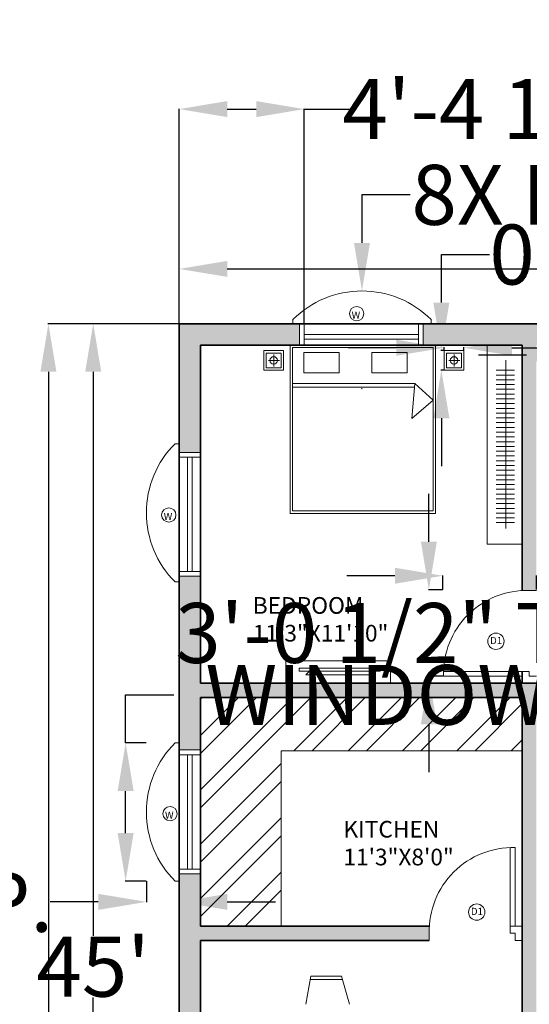
# Model space of a CAD drawing. Units: inches. Extents: x 28 to 3832, y 2 to 1709.
# Tile 3 of 7: x 2496 to 2710, y 1296 to 1709. Entities that reach past the tile are written whole.
import ezdxf

# ---------------------------------------------------------------- set-up
doc = ezdxf.new("R2010")
doc.units = ezdxf.units.IN
doc.header["$MEASUREMENT"] = 0
for name, color, linetype, lineweight in [('A-ANNO-DIMS', 2, 'Continuous', 18), ('A-ANNO-SYMB', 7, 'Continuous', 13), ('A-AREA-IDEN', 7, 'Continuous', 18), ('A-DOOR', 3, 'Continuous', 18), ('A-FLOR-CASE', 8, 'Continuous', 18), ('A-FLOR-CASE-PATT', 8, 'Continuous', 13), ('A-FLOR-FIXT', 9, 'Continuous', 18), ('A-FURN', 8, 'Continuous', 18), ('A-GLAZ', 4, 'Continuous', 18), ('A-ROOF-SHAD', 7, 'Continuous', 13), ('A-WALL', 7, 'Continuous', 35)]:
    doc.layers.add(name, color=color, linetype=linetype, lineweight=lineweight)
doc.layers.add('A-FLOR-FIXT-PATT', color=31, linetype='Continuous', lineweight=9, true_color=0xfecc66)
doc.layers.add('A-WALL-PATT', color=30, linetype='Continuous', lineweight=9, true_color=0xf26722)
doc.styles.get("Standard").update_dxf_attribs({"font": 'arial.ttf'})
doc.dimstyles.get("Standard").update_dxf_attribs({"dimtxt": 25.18, "dimasz": 20.18, "dimexe": 0.18, "dimexo": 0.0625, "dimgap": 0.09, "dimtad": 0, "dimtih": 1, "dimtoh": 1, "dimdec": 0, "dimzin": 0, "dimdsep": 46, "dimlunit": 3, "dimtxsty": 'Standard', "dimcen": 0.09, "dimadec": 0, "dimazin": 0, "dimtfac": 1, "dimtdec": 0, "dimtofl": 0, "dimtmove": 0, "dimatfit": 3, "dimfxl": 1, "dimtolj": 1, "dimtzin": 0, "dimarcsym": 0})

# ---------------------------------------------------------------- blocks, each defined once
blk = doc.blocks.new('*D1')
at = {"layer": 'A-ANNO-DIMS', "color": 0, "lineweight": -2, "transparency": 16777216}
for p, q in [((2562.64, 1581.59), (2562.64, 1604.74)), ((2582.82, 1604.56), (2721.19, 1604.56)), ((2902.46, 1604.56), (2764.09, 1604.56)), ((2922.64, 1581.59), (2922.64, 1604.74))]:
    blk.add_line(p, q, dxfattribs=at)
at = {"layer": 'A-ANNO-DIMS', "color": 0, "transparency": 16777216}
for points in [[(2582.82, 1607.92), (2582.82, 1601.2), (2562.64, 1604.56)], [(2902.46, 1607.92), (2902.46, 1601.2), (2922.64, 1604.56)]]:
    blk.add_solid(points, dxfattribs=at)
at = {"layer": 'Defpoints', "color": 0, "transparency": 16777216}
for p in [(2922.64, 1604.56), (2562.64, 1581.52), (2922.64, 1581.52)]:
    blk.add_point(p, dxfattribs=at)
at = {"layer": 'A-ANNO-DIMS', "color": 0, "transparency": 16777216, "insert": (2742.64, 1604.56), "char_height": 25.18, "attachment_point": 5}
blk.add_mtext("\\A1;30'", dxfattribs=at)
blk = doc.blocks.new('*D2')
at = {"layer": 'A-ANNO-DIMS', "color": 0, "lineweight": -2, "transparency": 16777216}
for p, q in [((2562.58, 1581.52), (2526.35, 1581.52)), ((2526.53, 1561.34), (2526.53, 1324.42)), ((2526.53, 1061.7), (2526.53, 1298.63)), ((2562.58, 1041.52), (2526.35, 1041.52))]:
    blk.add_line(p, q, dxfattribs=at)
at = {"layer": 'A-ANNO-DIMS', "color": 0, "transparency": 16777216}
for points in [[(2523.16, 1561.34), (2529.89, 1561.34), (2526.53, 1581.52)], [(2523.16, 1061.7), (2529.89, 1061.7), (2526.53, 1041.52)]]:
    blk.add_solid(points, dxfattribs=at)
at = {"layer": 'Defpoints', "color": 0, "transparency": 16777216}
for p in [(2562.64, 1581.52), (2526.53, 1041.52), (2562.64, 1041.52)]:
    blk.add_point(p, dxfattribs=at)
at = {"layer": 'A-ANNO-DIMS', "color": 0, "transparency": 16777216, "insert": (2526.53, 1311.52), "char_height": 25.18, "attachment_point": 5}
blk.add_mtext("\\A1;45'", dxfattribs=at)
blk = doc.blocks.new('DOOR-D1-36')
for p, q in [((33.01, 36), (39.01, 36)), ((36.01, 2), (0.01, 2)), ((33.01, 0), (0.01, 0)), ((36.01, 2), (36.01, 0)), ((36.01, 0), (39.01, 0))]:
    blk.add_line(p, q)
blk.add_arc((35.01, 1), 35.01, 88.3634, 181.6366)
blk = doc.blocks.new('WINDOW-48')
for p, q in [((0, 0), (0, 9)), ((2, 0), (2, 9)), ((50, 0), (50, 9)), ((52, 0), (52, 9)), ((2, 5.5), (50, 5.5)), ((2, 3.5), (50, 3.5))]:
    blk.add_line(p, q)
blk = doc.blocks.new('WINDOW-SHADE')
for p, q in [((0, 1.76), (0, 0)), ((58.03, 1.76), (58.03, 0))]:
    blk.add_line(p, q)
blk.add_arc((29.02, -27.22), 41.01, 44.9571, 135.0429)
blk = doc.blocks.new('CHAIR-DINING')
for p, q in [((0, 0), (2.18, 11.87)), ((1.91, 10.35), (15.39, 10.45)), ((2.18, 11.87), (14.98, 11.87)), ((14.98, 11.87), (18.42, 0))]:
    blk.add_line(p, q)
blk = doc.blocks.new('BEDSIDE-TABLE-SMALL')
for p, q in [((4.1, 6.52), (4.1, 1.57)), ((1.89, 4.09), (6.56, 4.09))]:
    blk.add_line(p, q)
for points in [[(0, 8.19), (8.2, 8.19), (8.2, 0), (0, 0)], [(1, 7.19), (7.2, 7.19), (7.2, 1), (1, 1)]]:
    blk.add_lwpolyline(points, close=True)
blk.add_circle((4.1, 4.09), 1.56)
blk = doc.blocks.new('OPENING-TAG-W')
blk.add_circle((3, 3), 3)
at = {"insert": (0.88, 3.88), "char_height": 3, "attachment_point": 1}
blk.add_mtext_dynamic_manual_height_columns('W', width=16.2124, gutter_width=1, heights=[0], dxfattribs=at)
blk = doc.blocks.new('OPENING-TAG-D1')
blk.add_circle((3.43, 3.43), 3.43)
at = {"insert": (0.97, 5.25), "char_height": 3, "attachment_point": 1}
blk.add_mtext_dynamic_manual_height_columns('D1', width=16.2124, gutter_width=1, heights=[0], dxfattribs=at)
blk = doc.blocks.new('*D23')
at = {"layer": 'A-ANNO-DIMS', "color": 0, "lineweight": -2, "transparency": 16777216}
for p, q in [((2540.14, 1405.47), (2540.14, 1425.65)), ((2540.14, 1425.65), (2560.32, 1425.65)), ((2548.79, 1405.47), (2539.96, 1405.47)), ((2540.14, 1367.62), (2540.14, 1385.29)), ((2548.79, 1347.44), (2539.96, 1347.44))]:
    blk.add_line(p, q, dxfattribs=at)
at = {"layer": 'A-ANNO-DIMS', "color": 0, "transparency": 16777216}
for points in [[(2536.78, 1385.29), (2543.51, 1385.29), (2540.14, 1405.47)], [(2536.78, 1367.62), (2543.51, 1367.62), (2540.14, 1347.44)]]:
    blk.add_solid(points, dxfattribs=at)
at = {"layer": 'Defpoints', "color": 0, "transparency": 16777216}
for p in [(2540.14, 1405.47), (2548.85, 1405.47), (2548.85, 1347.44)]:
    blk.add_point(p, dxfattribs=at)
at = {"layer": 'A-ANNO-DIMS', "color": 0, "transparency": 16777216, "insert": (2795, 1425.65), "char_height": 25.18, "attachment_point": 5}
blk.add_mtext('\\A1;WINDOW SHADE 4\'-10" TYP.', dxfattribs=at)
blk = doc.blocks.new('*D24')
at = {"layer": 'A-ANNO-DIMS', "color": 0, "lineweight": -2, "transparency": 16777216}
for p, q in [((2548.85, 1347.38), (2548.85, 1338.56)), ((2562.64, 1347.38), (2562.64, 1338.56)), ((2528.67, 1338.74), (2508.49, 1338.74)), ((2582.82, 1338.74), (2603, 1338.74))]:
    blk.add_line(p, q, dxfattribs=at)
at = {"layer": 'A-ANNO-DIMS', "color": 0, "transparency": 16777216}
for points in [[(2528.67, 1342.1), (2528.67, 1335.37), (2548.85, 1338.74)], [(2582.82, 1342.1), (2582.82, 1335.37), (2562.64, 1338.74)]]:
    blk.add_solid(points, dxfattribs=at)
at = {"layer": 'Defpoints', "color": 0, "transparency": 16777216}
for p in [(2548.85, 1347.44), (2562.64, 1347.44), (2548.85, 1338.74)]:
    blk.add_point(p, dxfattribs=at)
at = {"layer": 'A-ANNO-DIMS', "color": 0, "transparency": 16777216, "insert": (2432.84, 1338.74), "char_height": 25.18, "attachment_point": 5}
blk.add_mtext('\\A1;1\'-2" TYP.', dxfattribs=at)
blk = doc.blocks.new('*D27')
at = {"layer": 'A-ANNO-DIMS', "color": 0, "lineweight": -2, "transparency": 16777216}
for p, q in [((2616.64, 1234.6), (2616.64, 1231.72)), ((2635.06, 1234.6), (2635.06, 1231.72)), ((2596.46, 1231.9), (2576.28, 1231.9)), ((2655.24, 1231.9), (2675.42, 1231.9))]:
    blk.add_line(p, q, dxfattribs=at)
at = {"layer": 'A-ANNO-DIMS', "color": 0, "transparency": 16777216}
for points in [[(2596.46, 1235.27), (2596.46, 1228.54), (2616.64, 1231.9)], [(2655.24, 1235.27), (2655.24, 1228.54), (2635.06, 1231.9)]]:
    blk.add_solid(points, dxfattribs=at)
at = {"layer": 'Defpoints', "color": 0, "transparency": 16777216}
for p in [(2616.64, 1234.67), (2635.06, 1234.67), (2616.64, 1231.9)]:
    blk.add_point(p, dxfattribs=at)
at = {"layer": 'A-ANNO-DIMS', "color": 0, "transparency": 16777216, "insert": (2410.65, 1231.9), "char_height": 25.18, "attachment_point": 5}
blk.add_mtext('\\A1;CHAIR 1\'-6 1/2" TYP.', dxfattribs=at)
blk = doc.blocks.new('*D31')
at = {"layer": 'A-ANNO-DIMS', "color": 0, "lineweight": -2, "transparency": 16777216}
for p, q in [((2653.18, 1475.69), (2633, 1475.69)), ((2673.36, 1469.86), (2673.36, 1475.87)), ((2712.64, 1469.86), (2712.64, 1475.87)), ((2732.82, 1475.69), (2753, 1475.69))]:
    blk.add_line(p, q, dxfattribs=at)
at = {"layer": 'A-ANNO-DIMS', "color": 0, "transparency": 16777216}
for points in [[(2653.18, 1479.05), (2653.18, 1472.33), (2673.36, 1475.69)], [(2732.82, 1479.05), (2732.82, 1472.33), (2712.64, 1475.69)]]:
    blk.add_solid(points, dxfattribs=at)
at = {"layer": 'Defpoints', "color": 0, "transparency": 16777216}
for p in [(2712.64, 1475.69), (2673.36, 1469.8), (2712.64, 1469.8)]:
    blk.add_point(p, dxfattribs=at)
at = {"layer": 'A-ANNO-DIMS', "color": 0, "transparency": 16777216, "insert": (2943.56, 1475.69), "char_height": 25.18, "attachment_point": 5}
blk.add_mtext('\\A1;DOOR D1 3\'-3 1/2" TYP.', dxfattribs=at)
blk = doc.blocks.new('*D32')
at = {"layer": 'A-ANNO-DIMS', "color": 0, "lineweight": -2, "transparency": 16777216}
for p, q in [((2667.47, 1489.98), (2667.47, 1510.16)), ((2673.3, 1469.8), (2667.29, 1469.8)), ((2673.3, 1433.52), (2667.29, 1433.52)), ((2667.47, 1413.34), (2667.47, 1393.16))]:
    blk.add_line(p, q, dxfattribs=at)
at = {"layer": 'A-ANNO-DIMS', "color": 0, "transparency": 16777216}
for points in [[(2664.11, 1489.98), (2670.84, 1489.98), (2667.47, 1469.8)], [(2664.11, 1413.34), (2670.84, 1413.34), (2667.47, 1433.52)]]:
    blk.add_solid(points, dxfattribs=at)
at = {"layer": 'Defpoints', "color": 0, "transparency": 16777216}
for p in [(2667.47, 1469.8), (2673.36, 1469.8), (2673.36, 1433.52)]:
    blk.add_point(p, dxfattribs=at)
at = {"layer": 'A-ANNO-DIMS', "color": 0, "transparency": 16777216, "insert": (2667.47, 1451.66), "char_height": 25.18, "attachment_point": 5}
blk.add_mtext('\\A1;3\'-0 1/2" TYP.', dxfattribs=at)
blk = doc.blocks.new('*D35')
at = {"layer": 'A-ANNO-DIMS', "color": 0, "lineweight": -2, "transparency": 16777216}
for p, q in [((2728.64, 1572.46), (2728.64, 1568.14)), ((2756.64, 1572.46), (2756.64, 1568.14)), ((2708.46, 1568.32), (2688.28, 1568.32)), ((2776.82, 1568.32), (2797, 1568.32))]:
    blk.add_line(p, q, dxfattribs=at)
at = {"layer": 'A-ANNO-DIMS', "color": 0, "transparency": 16777216}
for points in [[(2708.46, 1571.69), (2708.46, 1564.96), (2728.64, 1568.32)], [(2776.82, 1571.69), (2776.82, 1564.96), (2756.64, 1568.32)]]:
    blk.add_solid(points, dxfattribs=at)
at = {"layer": 'Defpoints', "color": 0, "transparency": 16777216}
for p in [(2728.64, 1572.52), (2756.64, 1572.52), (2756.64, 1568.32)]:
    blk.add_point(p, dxfattribs=at)
at = {"layer": 'A-ANNO-DIMS', "color": 0, "transparency": 16777216, "insert": (2926.28, 1568.32), "char_height": 25.18, "attachment_point": 5}
blk.add_mtext('\\A1;VENT 2\'-4" TYP.', dxfattribs=at)
blk = doc.blocks.new('*D39')
at = {"layer": 'A-ANNO-DIMS', "color": 0, "lineweight": -2, "transparency": 16777216}
for p, q in [((2653.75, 1571.46), (2633.57, 1571.46)), ((2673.93, 1570.3), (2673.93, 1571.64)), ((2682.13, 1570.3), (2682.13, 1571.64)), ((2702.31, 1571.46), (2722.49, 1571.46))]:
    blk.add_line(p, q, dxfattribs=at)
at = {"layer": 'A-ANNO-DIMS', "color": 0, "transparency": 16777216}
for points in [[(2653.75, 1574.83), (2653.75, 1568.1), (2673.93, 1571.46)], [(2702.31, 1574.83), (2702.31, 1568.1), (2682.13, 1571.46)]]:
    blk.add_solid(points, dxfattribs=at)
at = {"layer": 'Defpoints', "color": 0, "transparency": 16777216}
for p in [(2682.13, 1571.46), (2673.93, 1570.23), (2682.13, 1570.23)]:
    blk.add_point(p, dxfattribs=at)
at = {"layer": 'A-ANNO-DIMS', "color": 0, "transparency": 16777216, "insert": (2981.04, 1571.46), "char_height": 25.18, "attachment_point": 5}
blk.add_mtext('\\A1;SMALL NIGHTSTAND 0\'-8" TYP.', dxfattribs=at)
blk = doc.blocks.new('*D40')
at = {"layer": 'A-ANNO-DIMS', "color": 0, "lineweight": -2, "transparency": 16777216}
for p, q in [((2672.7, 1590.41), (2672.7, 1610.59)), ((2672.7, 1610.59), (2692.88, 1610.59)), ((2673.87, 1570.23), (2672.52, 1570.23)), ((2673.87, 1562.04), (2672.52, 1562.04)), ((2672.7, 1541.86), (2672.7, 1521.68))]:
    blk.add_line(p, q, dxfattribs=at)
at = {"layer": 'A-ANNO-DIMS', "color": 0, "transparency": 16777216}
for points in [[(2669.34, 1590.41), (2676.07, 1590.41), (2672.7, 1570.23)], [(2669.34, 1541.86), (2676.07, 1541.86), (2672.7, 1562.04)]]:
    blk.add_solid(points, dxfattribs=at)
at = {"layer": 'Defpoints', "color": 0, "transparency": 16777216}
for p in [(2672.7, 1570.23), (2673.93, 1570.23), (2673.93, 1562.04)]:
    blk.add_point(p, dxfattribs=at)
at = {"layer": 'A-ANNO-DIMS', "color": 0, "transparency": 16777216, "insert": (2769.71, 1610.59), "char_height": 25.18, "attachment_point": 5}
blk.add_mtext('\\A1;0\'-8" TYP.', dxfattribs=at)
blk = doc.blocks.new('*D47')
at = {"layer": 'A-ANNO-DIMS', "color": 0, "lineweight": -2, "transparency": 16777216}
for p, q in [((2562.58, 1581.52), (2507.53, 1581.52)), ((2507.71, 1561.34), (2507.71, 1255.51)), ((2507.71, 923.79), (2507.71, 1229.62)), ((2634.1, 903.61), (2507.53, 903.61))]:
    blk.add_line(p, q, dxfattribs=at)
at = {"layer": 'A-ANNO-DIMS', "color": 0, "transparency": 16777216}
for points in [[(2504.35, 1561.34), (2511.07, 1561.34), (2507.71, 1581.52)], [(2504.35, 923.79), (2511.07, 923.79), (2507.71, 903.61)]]:
    blk.add_solid(points, dxfattribs=at)
at = {"layer": 'Defpoints', "color": 0, "transparency": 16777216}
for p in [(2507.71, 1581.52), (2562.64, 1581.52), (2634.16, 903.61)]:
    blk.add_point(p, dxfattribs=at)
at = {"layer": 'A-ANNO-DIMS', "color": 0, "transparency": 16777216, "insert": (2507.71, 1242.57), "char_height": 25.18, "attachment_point": 5}
blk.add_mtext('\\A1;56\'-6"', dxfattribs=at)
blk = doc.blocks.new('*D50')
at = {"layer": 'A-ANNO-DIMS', "color": 0, "lineweight": -2, "transparency": 16777216}
for p, q in [((2562.64, 1581.59), (2562.64, 1671.85)), ((2582.82, 1671.67), (2594.96, 1671.67)), ((2615.14, 1581.59), (2615.14, 1671.85)), ((2615.14, 1671.67), (2635.32, 1671.67))]:
    blk.add_line(p, q, dxfattribs=at)
at = {"layer": 'A-ANNO-DIMS', "color": 0, "transparency": 16777216}
for points in [[(2582.82, 1675.04), (2582.82, 1668.31), (2562.64, 1671.67)], [(2594.96, 1675.04), (2594.96, 1668.31), (2615.14, 1671.67)]]:
    blk.add_solid(points, dxfattribs=at)
at = {"layer": 'Defpoints', "color": 0, "transparency": 16777216}
for p in [(2615.14, 1671.67), (2562.64, 1581.52), (2615.14, 1581.52)]:
    blk.add_point(p, dxfattribs=at)
at = {"layer": 'A-ANNO-DIMS', "color": 0, "transparency": 16777216, "insert": (2698.72, 1671.67), "char_height": 25.18, "attachment_point": 5}
blk.add_mtext('\\A1;4\'-4 1/2"', dxfattribs=at)
blk = doc.blocks.new('*D67')
at = {"layer": 'A-ANNO-DIMS', "color": 0, "lineweight": -2, "transparency": 16777216}
for p, q in [((2659.56, 1635.67), (2639.38, 1635.67)), ((2639.38, 1635.67), (2639.38, 1615.49)), ((2639.29, 1554.31), (2639.47, 1554.31)), ((2639.38, 1554.22), (2639.38, 1554.4))]:
    blk.add_line(p, q, dxfattribs=at)
at = {"layer": 'A-ANNO-DIMS', "color": 0, "transparency": 16777216}
blk.add_solid([(2636.01, 1615.49), (2642.74, 1615.49), (2639.38, 1595.31)], dxfattribs=at)
at = {"layer": 'Defpoints', "color": 0, "transparency": 16777216}
for p in [(2639.38, 1595.31), (2639.38, 1554.31)]:
    blk.add_point(p, dxfattribs=at)
at = {"layer": 'A-ANNO-DIMS', "color": 0, "transparency": 16777216, "insert": (2732.23, 1635.67), "char_height": 25.18, "attachment_point": 5}
blk.add_mtext('\\A1;8X R3\'-5"', dxfattribs=at)

msp = doc.modelspace()

# ---------------------------------------------------------------- hatches: boundary and pattern name
at = {"layer": 'A-FLOR-CASE-PATT'}
h = msp.add_hatch(dxfattribs=at)
h.set_pattern_fill('ANSI31', color=256, scale=16, angle=-45, style=0)
h.paths.add_polyline_path([(2695.66, 1497.6), (2703.49, 1497.6), (2703.49, 1563.56), (2695.66, 1563.56)])
at = {"layer": 'A-FLOR-FIXT-PATT'}
h = msp.add_hatch(dxfattribs=at)
h.set_pattern_fill('ANSI32', color=256, scale=43)
h.paths.add_polyline_path([(2605.47, 1402.2), (2706.64, 1402.2), (2706.64, 1424.52), (2571.64, 1424.52), (2571.64, 1328.52), (2605.47, 1328.52)])
at = {"layer": 'A-WALL-PATT'}
h = msp.add_hatch(color=256, dxfattribs=at)
h.dxf.hatch_style = 1
h.paths.add_polyline_path([(2571.64, 1572.52), (2613.14, 1572.52), (2613.14, 1581.52), (2562.64, 1581.52), (2562.64, 1527.52), (2571.64, 1527.52)])
h.paths.add_polyline_path([(2728.64, 1581.52), (2665.14, 1581.52), (2665.14, 1572.52), (2670.22, 1572.52), (2706.64, 1572.52), (2706.64, 1469.52), (2707.64, 1469.52, -0.014283), (2709.64, 1469.52), (2712.64, 1469.52), (2712.64, 1471.52), (2712.64, 1477.52), (2712.64, 1572.52), (2728.64, 1572.52)])
h.paths.add_polyline_path([(2820.14, 1581.52), (2756.64, 1581.52), (2756.64, 1572.52), (2772.64, 1572.52), (2772.64, 1477.52), (2745.64, 1477.52), (2745.64, 1476.52, -0.017236), (2745.64, 1474.52), (2745.64, 1471.52), (2772.64, 1471.52), (2772.64, 1469.52), (2775.64, 1469.52, -0.006113), (2776.49, 1469.52), (2778.64, 1469.52), (2778.64, 1572.52), (2820.14, 1572.52)])
h.paths.add_polyline_path([(2922.64, 1581.52), (2872.14, 1581.52), (2872.14, 1572.52), (2913.64, 1572.52), (2913.64, 1527.52), (2922.64, 1527.52)])
h.paths.add_polyline_path([(2922.64, 1475.52), (2913.64, 1475.52), (2913.64, 1430.52), (2778.64, 1430.52), (2772.64, 1430.52), (2772.64, 1321.52), (2775.64, 1321.52, -0.014283), (2777.64, 1321.52), (2778.64, 1321.52), (2778.64, 1424.52), (2913.64, 1424.52), (2913.64, 1379.52), (2922.64, 1379.52)])
h.paths.add_polyline_path([(2571.64, 1475.52), (2562.64, 1475.52), (2562.64, 1402.52), (2571.64, 1402.52), (2571.64, 1424.52), (2706.64, 1424.52), (2706.64, 1328.52), (2706.64, 1322.52), (2706.64, 1290.16), (2712.64, 1290.16), (2712.64, 1430.52), (2706.64, 1430.52), (2571.64, 1430.52)])
h.paths.add_polyline_path([(2571.64, 1322.52), (2667.64, 1322.52), (2667.64, 1325.52, -0.014283), (2667.64, 1327.52), (2667.64, 1328.52), (2571.64, 1328.52), (2571.64, 1350.52), (2562.64, 1350.52), (2562.64, 1283.02), (2571.64, 1283.02)])
h.paths.add_polyline_path([(2712.64, 1241.01), (2706.64, 1241.01), (2706.64, 1191.52), (2571.64, 1191.52), (2571.64, 1231.02), (2562.64, 1231.02), (2562.64, 1172.52), (2571.64, 1172.52), (2571.64, 1185.52), (2706.64, 1185.52), (2712.64, 1185.52)])
h.paths.add_polyline_path([(2571.64, 1125.52), (2712.64, 1125.52), (2719.5, 1125.52), (2719.5, 1128.52), (2721.5, 1128.52), (2721.5, 1131.52), (2571.64, 1131.52), (2571.64, 1144.52), (2562.64, 1144.52), (2562.64, 1041.52), (2740.31, 1041.52), (2740.31, 1050.52), (2571.64, 1050.52)])
h.paths.add_polyline_path([(2712.64, 1152.52), (2709.64, 1152.52, -0.017236), (2707.64, 1152.52), (2706.64, 1152.52), (2706.64, 1131.52), (2712.64, 1131.52)])
h.paths.add_polyline_path([(2922.64, 1178.52), (2913.64, 1178.52), (2913.64, 1132.52), (2922.64, 1132.52)], flags=17)
h.paths.add_polyline_path([(2922.64, 1327.52), (2913.64, 1327.52), (2913.64, 1282.52), (2772.64, 1282.52), (2772.64, 1276.52), (2778.64, 1276.52), (2913.64, 1276.52), (2913.64, 1230.52), (2922.64, 1230.52)])
edge = h.paths.add_edge_path()
edge.add_line((2880.64, 1132.52), (2772.64, 1132.52))
edge.add_line((2772.64, 1132.52), (2772.64, 1126.52))
edge.add_line((2772.64, 1126.52), (2853.64, 1126.52))
edge.add_line((2853.64, 1126.52), (2853.64, 1050.52))
edge.add_line((2853.64, 1050.52), (2835.37, 1050.52))
edge.add_line((2835.37, 1050.52), (2835.37, 1041.52))
edge.add_line((2835.37, 1041.52), (2922.64, 1041.52))
edge.add_line((2922.64, 1041.52), (2922.64, 1074.52))
edge.add_line((2922.64, 1074.52), (2913.64, 1074.52))
edge.add_line((2913.64, 1074.52), (2913.64, 1050.52))
edge.add_line((2913.64, 1050.52), (2859.64, 1050.52))
edge.add_line((2859.64, 1050.52), (2859.64, 1126.52))
edge.add_line((2859.64, 1126.52), (2880.64, 1126.52))
edge.add_line((2880.64, 1126.52), (2880.64, 1127.52))
edge.add_arc((2909.64, 1128.52), 29.02, 178.0251, 181.9749, ccw=False)
edge.add_line((2880.64, 1129.52), (2880.64, 1132.52))

# ---------------------------------------------------------------- linework, layer by layer
at = {"layer": 'A-DOOR'}
for p, q in [((2701.64, 1328.52), (2706.64, 1328.52)), ((2703.64, 1322.52), (2706.64, 1322.52))]:
    msp.add_line(p, q, dxfattribs=at)
at = {"layer": 'A-FLOR-CASE'}
for p, q in [((2691.92, 1572.52), (2691.92, 1488.95)), ((2699.73, 1566.2), (2699.73, 1495.58)), ((2691.92, 1488.95), (2706.64, 1488.95))]:
    msp.add_line(p, q, dxfattribs=at)
at = {"layer": 'A-FLOR-FIXT'}
for p, q in [((2605.47, 1328.52), (2605.47, 1402.2)), ((2605.47, 1402.2), (2706.64, 1402.2))]:
    msp.add_line(p, q, dxfattribs=at)
at = {"layer": 'A-FURN'}
for p, q in [((2610.26, 1557.52), (2610.26, 1557.52)), ((2610.26, 1556.41), (2661.54, 1556.41)), ((2661.42, 1554.89), (2610.26, 1554.89)), ((2660.36, 1541.79), (2661.54, 1556.41)), ((2661.54, 1556.41), (2669.22, 1549.5)), ((2669.22, 1549.5), (2660.36, 1541.79)), ((2617.36, 1435.6), (2615.82, 1434.15)), ((2644.6, 1434.15), (2642.6, 1435.6)), ((2615.82, 1434.15), (2644.6, 1434.15))]:
    msp.add_line(p, q, dxfattribs=at)
for points in [[(2609.26, 1572.52), (2670.22, 1572.52), (2670.22, 1501.89), (2609.26, 1501.89)], [(2610.26, 1571.52), (2669.22, 1571.52), (2669.22, 1502.89), (2610.26, 1502.89)], [(2615.02, 1569.51), (2629.82, 1569.51), (2629.82, 1560.92), (2615.02, 1560.92)], [(2643.51, 1569.51), (2658.31, 1569.51), (2658.31, 1560.92), (2643.51, 1560.92)], [(2607.36, 1430.52), (2651.37, 1430.52), (2651.37, 1439.97), (2607.36, 1439.97)], [(2613.04, 1435.6), (2646.96, 1435.6), (2646.96, 1436.9), (2613.04, 1436.9)]]:
    msp.add_lwpolyline(points, close=True, dxfattribs=at)
at = {"layer": 'A-GLAZ'}
for p, q in [((2613.14, 1572.52), (2613.14, 1581.52)), ((2615.14, 1572.52), (2615.14, 1581.52)), ((2663.14, 1572.52), (2663.14, 1581.52)), ((2665.14, 1572.52), (2665.14, 1581.52)), ((2615.14, 1577.02), (2663.14, 1577.02)), ((2663.14, 1577.02), (2663.14, 1577.02)), ((2615.14, 1575.02), (2663.14, 1575.02))]:
    msp.add_line(p, q, dxfattribs=at)
at = {"layer": 'A-WALL'}
for p, q in [((2562.64, 1041.52), (2562.64, 1581.52)), ((2562.64, 1581.52), (2922.64, 1581.52)), ((2571.64, 1572.52), (2706.64, 1572.52)), ((2571.64, 1430.52), (2571.64, 1572.52)), ((2706.64, 1469.48), (2706.64, 1572.52)), ((2706.64, 1469.48), (2706.64, 1572.52)), ((2706.64, 1430.52), (2706.64, 1435.52)), ((2706.64, 1430.52), (2706.64, 1435.52)), ((2571.64, 1430.52), (2706.64, 1430.52)), ((2706.64, 1430.52), (2712.64, 1430.52)), ((2571.64, 1424.52), (2706.64, 1424.52)), ((2571.64, 1328.52), (2571.64, 1424.52)), ((2706.64, 1328.52), (2706.64, 1424.52)), ((2571.64, 1328.52), (2667.68, 1328.52)), ((2706.64, 1328.52), (2706.64, 1322.52)), ((2571.64, 1322.52), (2667.64, 1322.52)), ((2571.64, 1191.52), (2571.64, 1322.52)), ((2706.64, 1290.16), (2706.64, 1322.52))]:
    msp.add_line(p, q, dxfattribs=at)

# ---------------------------------------------------------------- block references
at = {"layer": 'A-ANNO-SYMB'}
for name, p in [('OPENING-TAG-W', (2634.16, 1582.78)), ('OPENING-TAG-W', (2555.26, 1498.21)), ('OPENING-TAG-D1', (2692.19, 1444.74)), ('OPENING-TAG-W', (2555.8, 1372.77)), ('OPENING-TAG-D1', (2684.14, 1331))]:
    msp.add_blockref(name, p, dxfattribs=at)
at = {"layer": 'A-DOOR'}
msp.add_blockref('DOOR-D1-36', (2673.62, 1433.52), dxfattribs=at)
at = {"layer": 'A-DOOR', "extrusion": (0, 0, -1), "zscale": -1, "rotation": 269.9999999999982}
msp.add_blockref('DOOR-D1-36', (-2703.64, 1361.54), dxfattribs=at)
at = {"layer": 'A-FURN'}
for name, p in [('BEDSIDE-TABLE-SMALL', (2598.2, 1562.04)), ('BEDSIDE-TABLE-SMALL', (2673.93, 1562.04)), ('CHAIR-DINING', (2615.76, 1295.72))]:
    msp.add_blockref(name, p, dxfattribs=at)
at = {"layer": 'A-GLAZ'}
for p, rotation in [((2571.64, 1475.52), 90.00000000000081), ((2571.64, 1350.52), 90.00000000000072)]:
    msp.add_blockref('WINDOW-48', p, dxfattribs=dict(at, rotation=rotation))
at = {"layer": 'A-ROOF-SHAD'}
msp.add_blockref('WINDOW-SHADE', (2610.36, 1581.52), dxfattribs=at)
for p, rotation in [((2562.64, 1473.11), 90.00000000001451), ((2562.64, 1347.44), 90.00000000001474)]:
    msp.add_blockref('WINDOW-SHADE', p, dxfattribs=dict(at, rotation=rotation))

# ---------------------------------------------------------------- texts
at = {"layer": 'A-AREA-IDEN', "char_height": 7, "attachment_point": 1}
for s, insert in [('BEDROOM\\P11\'3"X11\'10"', (2593.52, 1466.73)), ('KITCHEN\\P11\'3"X8\'0"', (2631.58, 1372.74))]:
    msp.add_mtext_dynamic_manual_height_columns(s, width=107.6964, gutter_width=1, heights=[0], dxfattribs=dict(at, insert=insert))

# ---------------------------------------------------------------- dimensions: what is measured, and where the dimension line sits
at = {"layer": 'A-ANNO-DIMS'}
for base, p2, override, picture, middle in [((2615.14, 1671.67), (2615.14, 1581.52), {"dimdec": 1, "dimlfac": 1, "dimrnd": 0, "dimzin": 1, "dimdsep": 46, "dimlunit": 4, "dimfrac": 2}, '*D50', (2698.72, 1671.67)), ((2922.64, 1604.56), (2922.64, 1581.52), {"dimclrd": 0, "dimclre": 0, "dimclrt": 0}, '*D1', (2742.64, 1604.56))]:
    dim = msp.add_linear_dim(base=base, p1=(2562.64, 1581.52), p2=p2, dimstyle='Standard', override=override, dxfattribs=at)
    dim.commit()
    dim.dimension.update_dxf_attribs({"geometry": picture, "text_midpoint": middle})
dim = msp.add_radius_dim(center=(2639.38, 1554.31), mpoint=(2639.38, 1595.31), text='8X <>', dimstyle='Standard', override={"dimdec": 1, "dimlfac": 1, "dimrnd": 0, "dimzin": 1, "dimdsep": 46, "dimlunit": 4, "dimfrac": 2}, dxfattribs=at)
dim.commit()
dim.dimension.update_dxf_attribs({"geometry": '*D67', "text_midpoint": (2732.23, 1635.67)})
for base, p1, p2, text, picture, middle in [((2682.13, 1571.46), (2673.93, 1570.23), (2682.13, 1570.23), 'SMALL NIGHTSTAND <> TYP.', '*D39', (2981.04, 1571.46)), ((2756.64, 1568.32), (2728.64, 1572.52), (2756.64, 1572.52), 'VENT <> TYP.', '*D35', (2926.28, 1568.32)), ((2712.64, 1475.69), (2673.36, 1469.8), (2712.64, 1469.8), 'DOOR D1 <> TYP.', '*D31', (2943.56, 1475.69))]:
    dim = msp.add_linear_dim(base=base, p1=p1, p2=p2, text=text, dimstyle='Standard', override={"dimdec": 1, "dimlfac": 1, "dimrnd": 0, "dimzin": 1, "dimdsep": 46, "dimlunit": 4, "dimfrac": 2}, dxfattribs=at)
    dim.commit()
    dim.dimension.update_dxf_attribs({"geometry": picture, "text_midpoint": middle})
for base, p1, p2, angle, text, picture, middle in [((2672.7, 1570.23), (2673.93, 1562.04), (2673.93, 1570.23), 90, '<> TYP.', '*D40', (2769.71, 1610.59)), ((2667.47, 1469.8), (2673.36, 1433.52), (2673.36, 1469.8), 90, '<> TYP.', '*D32', (2667.47, 1451.66)), ((2540.14, 1405.47), (2548.85, 1347.44), (2548.85, 1405.47), 90, 'WINDOW SHADE <> TYP.', '*D23', (2795, 1425.65)), ((2548.85, 1338.74), (2562.64, 1347.44), (2548.85, 1347.44), 180, '<> TYP.', '*D24', (2432.84, 1338.74)), ((2616.64, 1231.9), (2635.06, 1234.67), (2616.64, 1234.67), 180, 'CHAIR <> TYP.', '*D27', (2410.65, 1231.9))]:
    dim = msp.add_linear_dim(base=base, p1=p1, p2=p2, angle=angle, text=text, dimstyle='Standard', override={"dimdec": 1, "dimlfac": 1, "dimrnd": 0, "dimzin": 1, "dimdsep": 46, "dimlunit": 4, "dimfrac": 2}, dxfattribs=at)
    dim.commit()
    dim.dimension.update_dxf_attribs({"geometry": picture, "text_midpoint": middle})
for base, p1, p2, override, picture, middle in [((2507.71, 1581.52), (2634.16, 903.61), (2562.64, 1581.52), {"dimdec": 1, "dimlfac": 1, "dimrnd": 0, "dimzin": 1, "dimdsep": 46, "dimlunit": 4, "dimfrac": 2}, '*D47', (2507.71, 1242.57)), ((2526.53, 1041.52), (2562.64, 1581.52), (2562.64, 1041.52), {"dimclrd": 0, "dimclre": 0, "dimclrt": 0}, '*D2', (2526.53, 1311.52))]:
    dim = msp.add_linear_dim(base=base, p1=p1, p2=p2, angle=90, dimstyle='Standard', override=override, dxfattribs=at)
    dim.commit()
    dim.dimension.update_dxf_attribs({"geometry": picture, "text_midpoint": middle})

doc.saveas('drawing.dxf')
